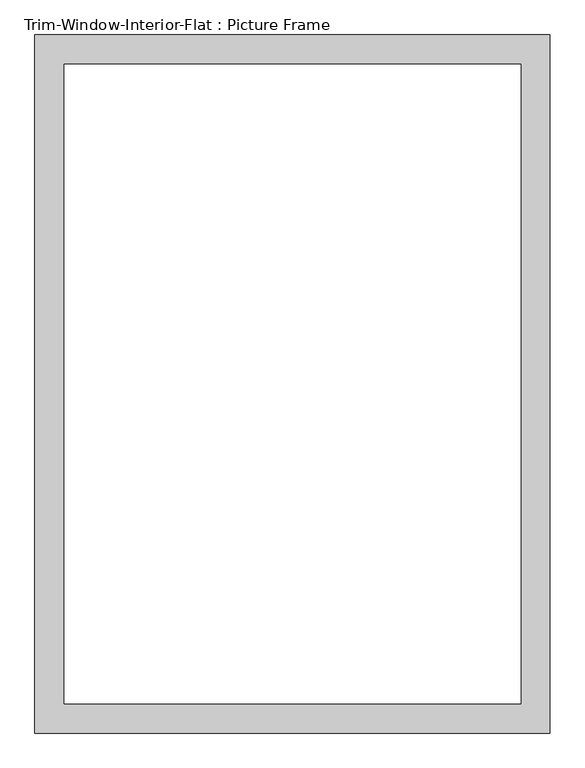
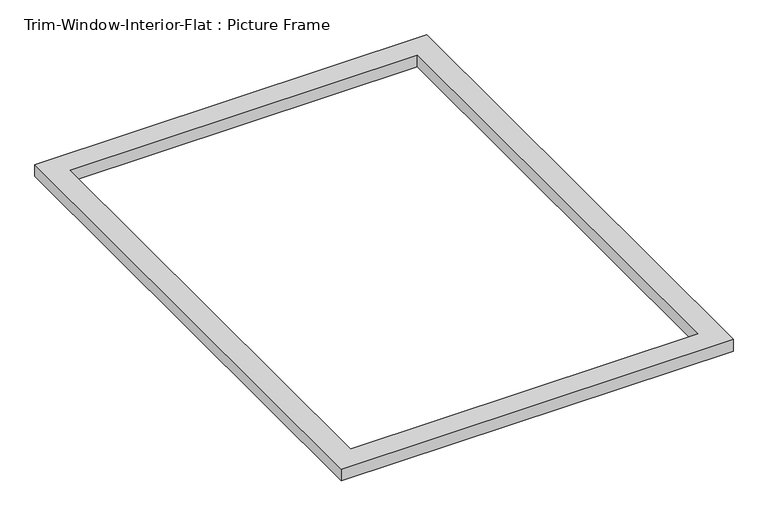
"""IFC4 building model written with IfcOpenShell, lengths in millimetres: proxy geometry, Trim-Window-Interior-Flat : Picture Frame."""

from ifc_helpers import new_model, si_unit, origin, origin_with_axes, place, context, project, spatial, polyline, outline, extrude, source, transform, mapped, element, save


def trim_window_interior_flat_picture_frame_e50cf7ae(model_context):
    return source(origin(), model_context, "Body", "SweptSolid", [
        extrude(outline(polyline([(501.65, 44.45), (501.65, -1314.45), (-501.65, -1314.45), (-501.65, 44.45), (501.65, 44.45)]), holes=[polyline([(444.5, -12.7), (-444.5, -12.7), (-444.5, -1257.3), (444.5, -1257.3), (444.5, -12.7)])]), origin_with_axes(), (0.0, 0.0, 1.0), 31.75),
    ])


if __name__ == "__main__":
    model = new_model("IFC4")
    model_context = context("Model", 3, world=origin())
    ifc_project = project(units=[si_unit("LENGTHUNIT", "METRE", prefix="MILLI")], contexts=[model_context])
    site = spatial("IfcSite", under=ifc_project)
    building = spatial("IfcBuilding", under=site)
    placement = place(None, origin())
    trim_window_interior_flat_picture_frame_shape = trim_window_interior_flat_picture_frame_e50cf7ae(model_context)
    element("IfcBuildingElementProxy", 1, Name="Trim-Window-Interior-Flat : Picture Frame", ObjectType="Trim-Window-Interior-Flat : Picture Frame", at=placement, inside=building, context=model_context, shape_type="MappedRepresentation", body=[
        mapped(trim_window_interior_flat_picture_frame_shape, transform((0.0, 0.0, 0.0), x_axis=(1.0, 0.0, 0.0), y_axis=(0.0, 1.0, 0.0), z_axis=(0.0, 0.0, 1.0))),
    ])
    save(model, "model.ifc")

# Revit data of these elements
# Type "Trim-Window-Interior-Flat : Picture Frame"
#   Trim Thickness_Picture Frame = 0' - 1 1/4"
#   Trim Width = 0' - 2 1/4"
#   Trim Thickness_with Sill = 0' - 0 3/4"
#   Sill Thickness = 0' - 1 1/4"
#   Opening Width [instance default] = 2' - 0"
#   Opening Height [instance default] = 3' - 0"
#   Default Elevation = 4' - 0"
#   Sill = no
#   Picture Frame = yes
#   Trim Material [instance default] = none
# Element 1 (IfcBuildingElementProxy, "Trim-Window-Interior-Flat : Picture Frame")
#   Opening Width = 3' - 0"
#   Opening Height = 4' - 2"
#   Trim Material = Wood - Stained
#   Materials on its faces: "Wood - Stained"
# Materials
#   "Wood - Stained": class "Wood", colour RGB 224 178 126, transparency 0, Cost = 0
